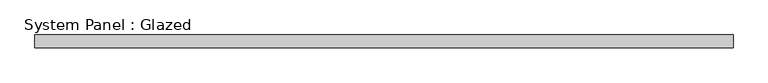
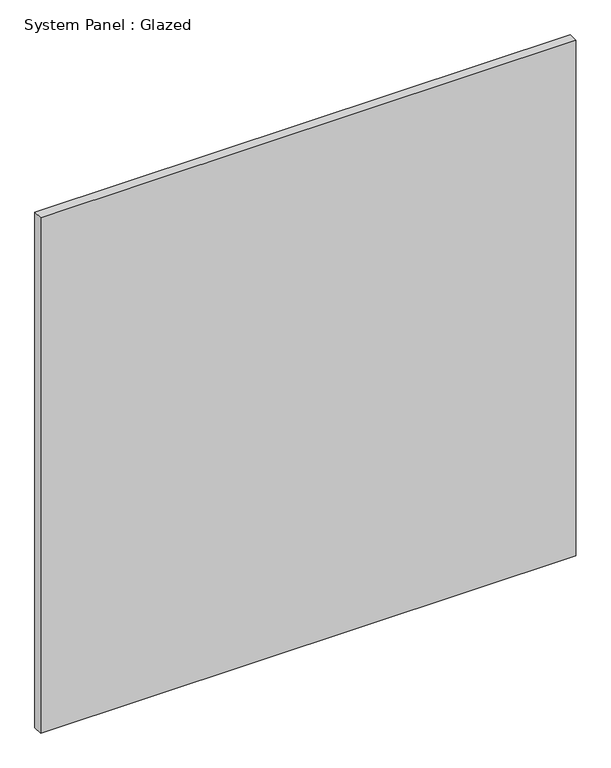
"""IFC4 building model written with IfcOpenShell, lengths in millimetres: plate geometry, System Panel : Glazed."""

from ifc_helpers import new_model, si_unit, origin, origin_with_axes, place, context, project, spatial, polyline, outline, extrude, source, transform, mapped, element, save


def system_panel_glazed_0f0a4f2b(model_context):
    return source(origin(), model_context, "Body", "SweptSolid", [
        extrude(outline(polyline([(701.6749999, -44.45), (-701.6749999, -44.45), (-701.6749999, -19.05), (701.6749999, -19.05), (701.6749999, -44.45)])), origin_with_axes(), (0.0, 0.0, 1.0), 1428.75),
    ])


if __name__ == "__main__":
    model = new_model("IFC4")
    model_context = context("Model", 3, world=origin())
    ifc_project = project(units=[si_unit("LENGTHUNIT", "METRE", prefix="MILLI")], contexts=[model_context])
    site = spatial("IfcSite", under=ifc_project)
    building = spatial("IfcBuilding", under=site)
    placement = place(None, origin())
    system_panel_glazed_shape = system_panel_glazed_0f0a4f2b(model_context)
    element("IfcPlate", 1, ObjectType="System Panel : Glazed", at=placement, inside=building, context=model_context, shape_type="MappedRepresentation", body=[
        mapped(system_panel_glazed_shape, transform((0.0, 0.0, 0.0), x_axis=(1.0, 0.0, 0.0), y_axis=(0.0, 1.0, 0.0), z_axis=(0.0, 0.0, 1.0))),
    ])
    save(model, "model.ifc")

# Revit data of these elements
# Type "System Panel : Glazed"
#   Construction Type Id = "GSP4R"
#   Analytic Construction = "1/8 in Pilkington single glazing"
#   Visual Light Transmittance = 0.9
#   Solar Heat Gain Coefficient = 0.86
#   Heat Transfer Coefficient (U) = 1.18115 BTU/(h·ft²·°F)
#   Define Thermal Properties by = 1
# Element 1 (IfcPlate, "System Panel : Glazed")
#   Materials on its faces: "Glass"
# Materials
#   "Glass": class "Glass", colour RGB 0 128 192, transparency 0.75, Description = "Soda Lime Glass", Cost = 0
